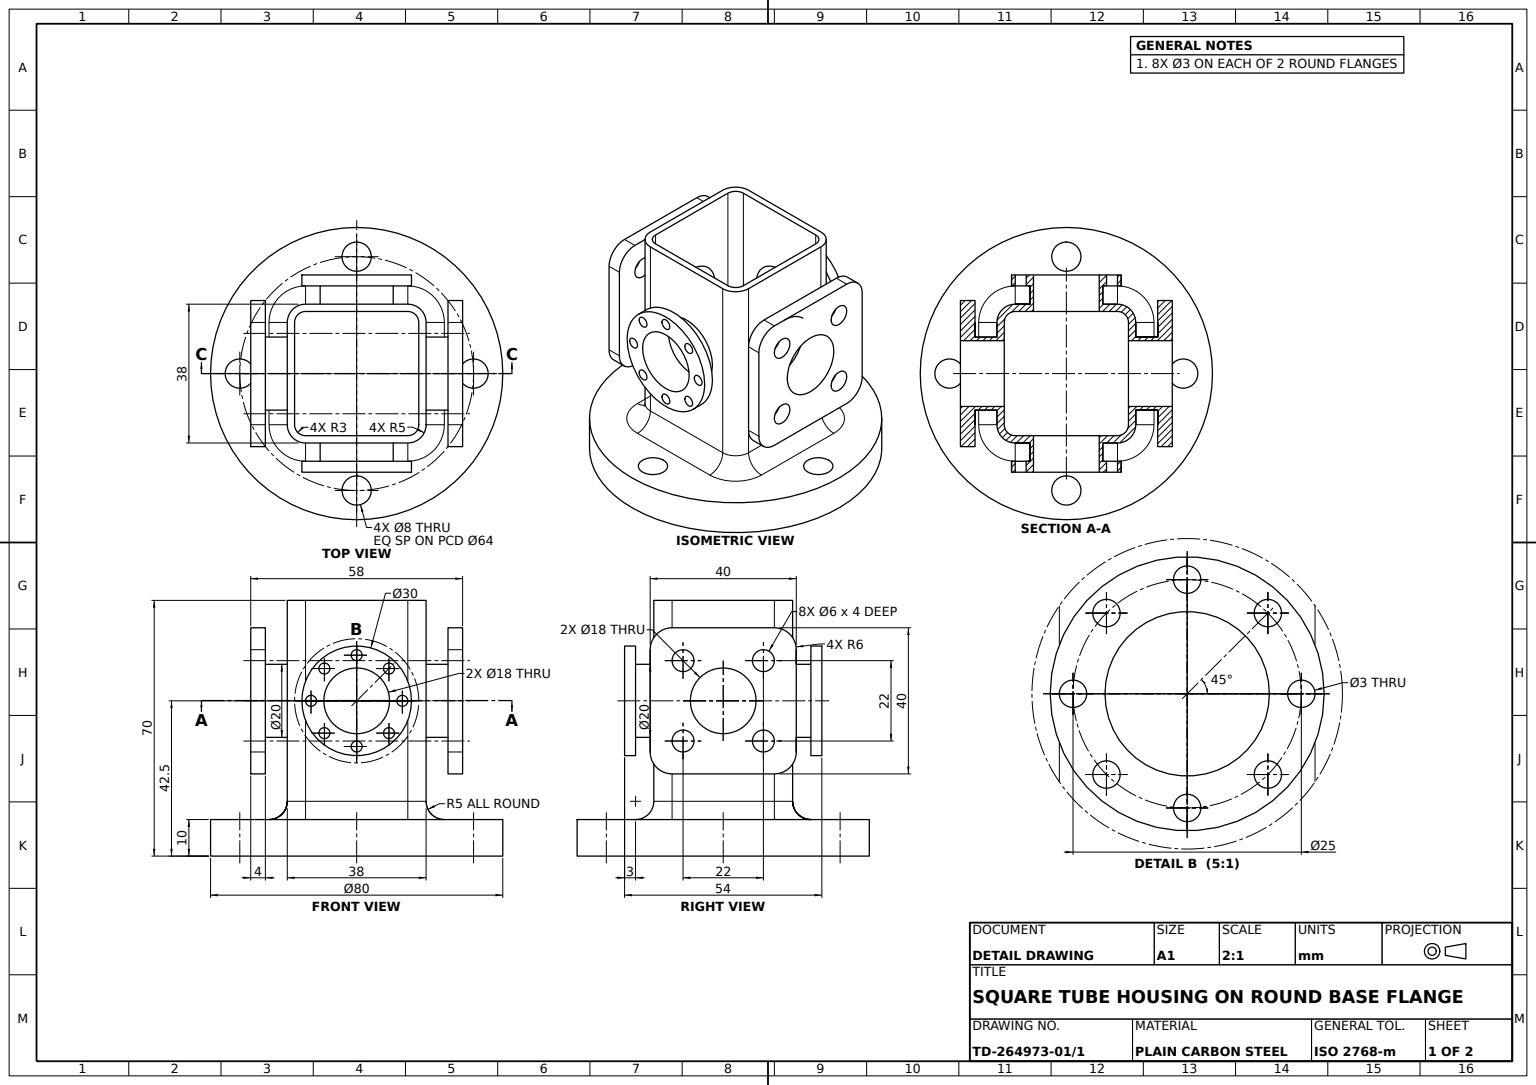
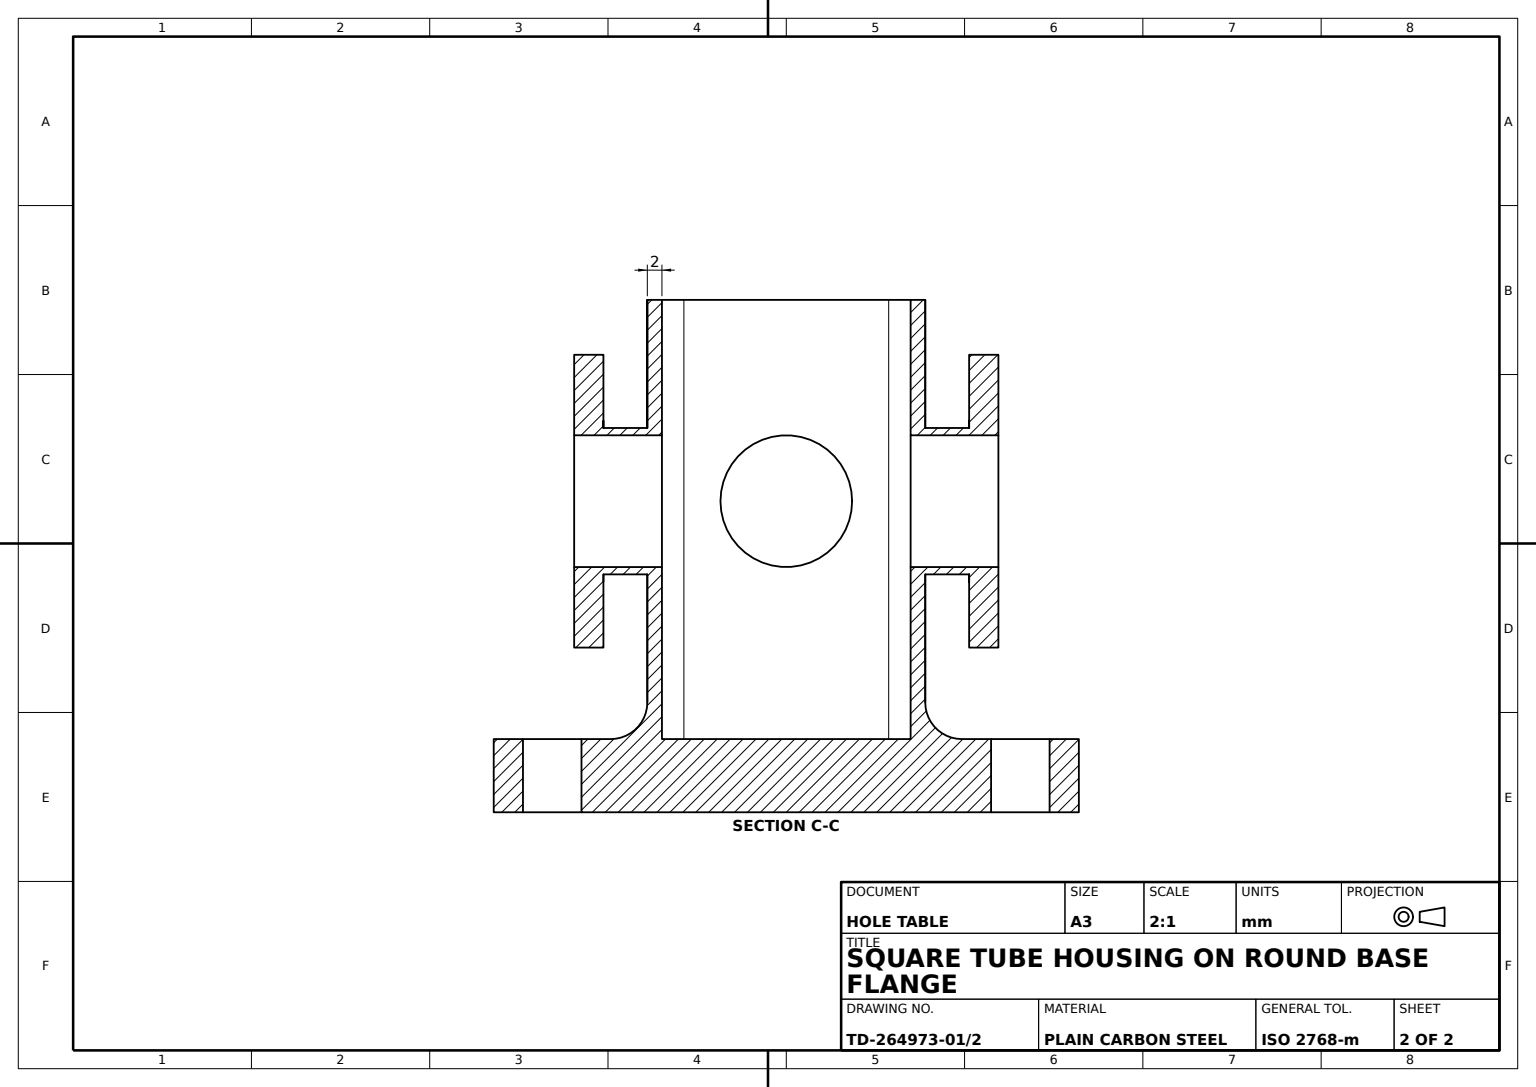
SolidWorks part; units mm, degrees
material "Plain Carbon Steel"
ref_plane "Front Plane" through (0, 0, 0) normal (0, 0, 1) x (1, 0, 0)
ref_plane "Top Plane" through (0, 0, 0) normal (0, 1, 0) x (1, 0, 0)
ref_plane "Right Plane" through (0, 0, 0) normal (1, 0, 0) x (0, 0, -1)
sketch "Base Flange Sketch" plane through (0, 0, 0) normal (0, 1, 0) x (1, 0, 0)
  circle A0 centre (0, 0) radius 40
  circle A2 centre (0, 32) radius 4
  circle A3 centre (32, 0) radius 4
  circle A4 centre (0, -32) radius 4
  circle A5 centre (-32, 0) radius 4
  dimension "D1" = 80
  dimension "D2" = 32
  dimension "D3" = 8
extrude "Base Flange Ø80" add sketch "Base Flange Sketch" along normal blind 10
sketch "Square Body Sketch" plane through (0, 10, 0) normal (0, 1, 0) x (1, 0, 0)
  line L1 (-14, 19) -> (14, 19)
  line L2 (-19, 14) -> (-19, -14)
  line L3 (-14, -19) -> (14, -19)
  line L4 (19, 14) -> (19, -14)
  line L5 (-19, 19) -> (19, -19) construction
  line L6 (-19, -19) -> (19, 19) construction
  arc A0 (14, -19) -> (19, -14) centre (14, -14) ccw
  arc A1 (-19, -14) -> (-14, -19) centre (-14, -14) ccw
  arc A2 (-14, 19) -> (-19, 14) centre (-14, 14) ccw
  arc A3 (14, 19) -> (19, 14) centre (14, 14) cw
  point P0 (0, 0)
  dimension "D2" = 5
  dimension "D1" = 38
extrude "Square Body 38x38 Wall 2" add sketch "Square Body Sketch" along normal blind 60 thin
fillet "Body to Flange Fillet R5" radius 5 8 edges at (-17.5355, 10, 17.5355) (-19, 10, 0) (-17.5355, 10, -17.5355) (0, 10, -19) (17.5355, 10, -17.5355) (19, 10, 0) (17.5355, 10, 17.5355) (0, 10, 19)
sketch "Cross Bore A Sketch" plane through (0, 0, 19) normal (0, 0, 1) x (1, 0, 0)
  line L0 (14, 70) -> (14, 15) construction
  line L1 (-14, 70) -> (14, 70) construction
  circle A0 centre (0, 42.5) radius 9
  dimension "D1" = 18
  dimension "D2" = 14
  dimension "D3" = 27.5
extrude "Cross Bore A Ø18" cut sketch "Cross Bore A Sketch" against normal blind 60
sketch "Cross Bore B Sketch" plane through (-19, 0, 0) normal (-1, 0, 0) x (0, 0, 1)
  line L0 (14, 70) -> (14, 15) construction
  line L1 (-14, 70) -> (14, 70) construction
  circle A0 centre (0, 42.5) radius 9
  dimension "D1" = 18
  dimension "D2" = 14
  dimension "D3" = 27.5
extrude "Cross Bore B Ø18" cut sketch "Cross Bore B Sketch" against normal blind 60
sketch "Port A1 Stub Sketch" plane through (0, 0, 19) normal (0, 0, 1) x (1, 0, 0)
  circle A0 centre (0, 42.5) radius 9
  dimension "D1" = 18
extrude "Port A1 Stub Ø18" add sketch "Port A1 Stub Sketch" along normal blind 5 thin
sketch "Round Flange A1 Sketch" plane through (0, 0, 24) normal (0, 0, 1) x (1, 0, 0)
  circle A0 centre (0, 42.5) radius 9
  circle A1 centre (0, 42.5) radius 15
  circle A3 centre (0, 55) radius 1.5
  circle A4 centre (8.8388, 51.3388) radius 1.5
  circle A5 centre (12.5, 42.5) radius 1.5
  circle A6 centre (8.8388, 33.6612) radius 1.5
  circle A7 centre (0, 30) radius 1.5
  circle A8 centre (-8.8388, 33.6612) radius 1.5
  circle A9 centre (-12.5, 42.5) radius 1.5
  circle A10 centre (-8.8388, 51.3388) radius 1.5
  circle A11 centre (0, 42.5) radius 10 construction
  dimension "D1" = 18
  dimension "D2" = 30
  dimension "D3" = 3
  dimension "D4" = 8.8388
extrude "Round Flange A1 Ø30" add sketch "Round Flange A1 Sketch" along normal blind 3
sketch "Port A2 Stub Sketch" plane through (0, 0, -19) normal (0, 0, -1) x (-1, 0, 0)
  circle A0 centre (0, 42.5) radius 9
  dimension "D1" = 18
extrude "Port A2 Stub Ø18" add sketch "Port A2 Stub Sketch" along normal blind 5 thin
sketch "Round Flange A2 Sketch" plane through (0, 0, -24) normal (0, 0, -1) x (-1, 0, 0)
  circle A0 centre (0, 42.5) radius 9
  circle A1 centre (0, 42.5) radius 15
  circle A3 centre (0, 55) radius 1.5
  circle A4 centre (8.8388, 51.3388) radius 1.5
  circle A5 centre (12.5, 42.5) radius 1.5
  circle A6 centre (8.8388, 33.6612) radius 1.5
  circle A7 centre (0, 30) radius 1.5
  circle A8 centre (-8.8388, 33.6612) radius 1.5
  circle A9 centre (-12.5, 42.5) radius 1.5
  circle A10 centre (-8.8388, 51.3388) radius 1.5
  circle A11 centre (0, 42.5) radius 10 construction
  dimension "D1" = 30
  dimension "D2" = 18
  dimension "D3" = 3
  dimension "D4" = 8.8388
extrude "Round Flange A2 Ø30" add sketch "Round Flange A2 Sketch" along normal blind 3
sketch "Port B1 Stub Sketch" plane through (-19, 0, 0) normal (-1, 0, 0) x (0, 0, 1)
  circle A0 centre (0, 42.5) radius 9
  dimension "D1" = 18
extrude "Port B1 Stub Ø18" add sketch "Port B1 Stub Sketch" along normal blind 6 thin
sketch "Square Flange B1 Sketch" plane through (-25, 0, 0) normal (-1, 0, 0) x (0, 0, 1)
  line L0 (14, 70) -> (14, 15) construction
  line L2 (-14, 62.5) -> (14, 62.5)
  line L3 (-20, 56.5) -> (-20, 28.5)
  line L4 (-14, 22.5) -> (14, 22.5)
  line L5 (20, 56.5) -> (20, 28.5)
  line L6 (-20, 62.5) -> (20, 22.5) construction
  line L7 (-20, 22.5) -> (20, 62.5) construction
  arc A0 (-20, 28.5) -> (-14, 22.5) centre (-14, 28.5) ccw
  arc A1 (14, 22.5) -> (20, 28.5) centre (14, 28.5) ccw
  arc A2 (14, 62.5) -> (20, 56.5) centre (14, 56.5) cw
  arc A3 (-14, 62.5) -> (-20, 56.5) centre (-14, 56.5) ccw
  circle A4 centre (0, 42.5) radius 9
  circle A5 centre (-11, 53.5) radius 3
  circle A6 centre (11, 53.5) radius 3
  circle A7 centre (-11, 31.5) radius 3
  circle A8 centre (11, 31.5) radius 3
  point P0 (0, 42.5)
  point P4 (0, 42.5)
  dimension "D4" = 6
  dimension "D5" = 18
  dimension "D6" = 6
  dimension "D7" = 6
  dimension "D8" = 6
  dimension "D9" = 6
  dimension "D1" = 40
  dimension "D2" = 42.5
  dimension "D3" = 14
  dimension "D10" = 9
  dimension "D11" = 9
  dimension "D12" = 9
  dimension "D13" = 9
extrude "Square Flange B1 40x40" add sketch "Square Flange B1 Sketch" along normal blind 4
sketch "Port B2 Stub Sketch" plane through (19, 0, 0) normal (1, 0, 0) x (0, 0, -1)
  circle A0 centre (0, 42.5) radius 9
  dimension "D1" = 18
extrude "Port B2 Stub Ø18" add sketch "Port B2 Stub Sketch" along normal blind 6 thin
sketch "Square Flange B2 Sketch" plane through (25, 0, 0) normal (1, 0, 0) x (0, 0, -1)
  line L1 (-14, 62.5) -> (14, 62.5)
  line L2 (-20, 56.5) -> (-20, 28.5)
  line L3 (-14, 22.5) -> (14, 22.5)
  line L4 (20, 56.5) -> (20, 28.5)
  line L5 (-20, 62.5) -> (20, 22.5) construction
  line L6 (-20, 22.5) -> (20, 62.5) construction
  circle A0 centre (0, 42.5) radius 9
  arc A1 (-20, 28.5) -> (-14, 22.5) centre (-14, 28.5) ccw
  arc A2 (14, 22.5) -> (20, 28.5) centre (14, 28.5) ccw
  arc A3 (14, 62.5) -> (20, 56.5) centre (14, 56.5) cw
  arc A4 (-14, 62.5) -> (-20, 56.5) centre (-14, 56.5) ccw
  circle A5 centre (-11, 53.5) radius 3
  circle A6 centre (-11, 31.5) radius 3
  circle A7 centre (11, 31.5) radius 3
  circle A8 centre (11, 53.5) radius 3
  dimension "D1" = 40
  dimension "D2" = 18
  dimension "D3" = 6
  dimension "D4" = 6
  dimension "D5" = 6
  dimension "D6" = 6
  dimension "D7" = 6
  dimension "D8" = 9
  dimension "D9" = 9
  dimension "D10" = 9
  dimension "D11" = 9
extrude "Square Flange B2 40x40" add sketch "Square Flange B2 Sketch" along normal blind 4
